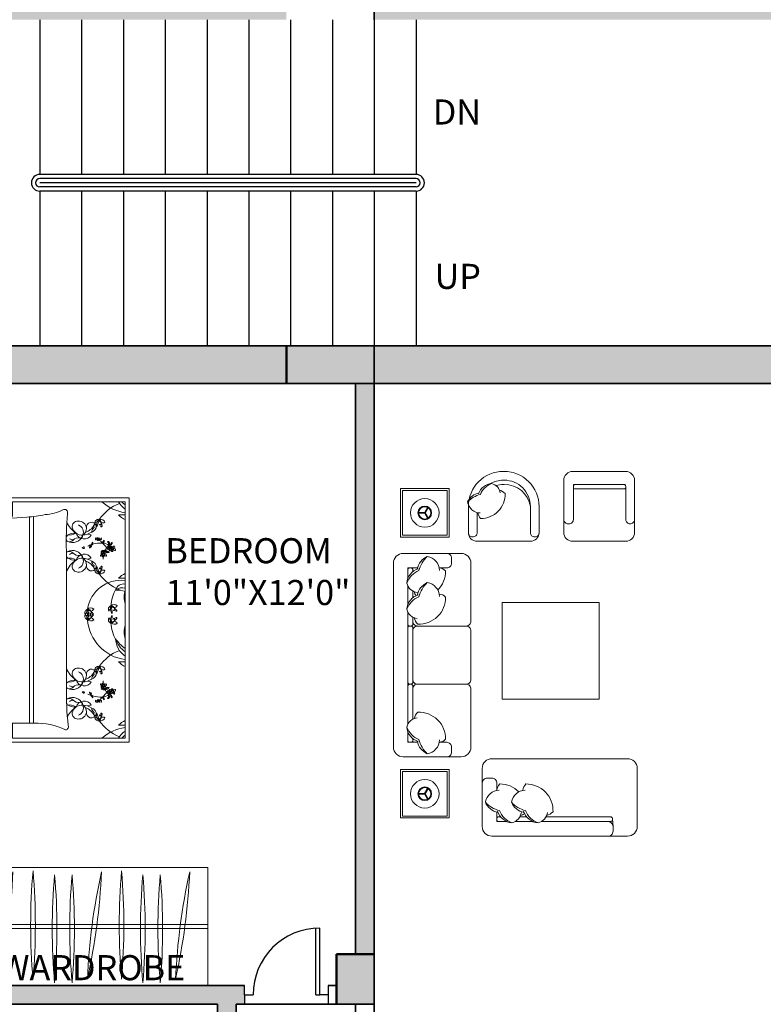
# Model space of a CAD drawing. Units: inches. Extents: x -28 to 485, y -861 to 54.
# Tile 3 of 14: x 76 to 254, y -600 to -365. Entities that reach past the tile are written whole.
import ezdxf

# ---------------------------------------------------------------- set-up
doc = ezdxf.new("R2010")
doc.units = ezdxf.units.IN
doc.header["$MEASUREMENT"] = 0
for name, color, linetype, lineweight in [('A-ANNO-TEXT', 7, 'Continuous', 18), ('A-AREA-IDEN', 7, 'Continuous', 18), ('A-COLS', 7, 'Continuous', 50), ('A-COLS-PATT', 8, 'Continuous', 13), ('A-DOOR', 3, 'Continuous', 25), ('A-FLOR-CASE', 8, 'Continuous', 18), ('A-FLOR-STRS', 7, 'Continuous', 25), ('A-FURN', 8, 'Continuous', 13), ('A-WALL', 7, 'Continuous', 35), ('A-WALL-PATT', 34, 'Continuous', 13)]:
    doc.layers.add(name, color=color, linetype=linetype, lineweight=lineweight)
doc.styles.get("Standard").update_dxf_attribs({"font": 'arial.ttf'})

# ---------------------------------------------------------------- blocks, each defined once
blk = doc.blocks.new('DAY BED1')
at = {"color": 0}
blk.add_line((0.3, 0.25), (0.225, 0.255), dxfattribs=at)
blk.add_lwpolyline([(-0.3, 0, -0.414214), (-0.4, 0.1), (-0.4, 0.1, 0.317837), (-0.4, 0.1, -0.414214), (-0.4, 0.1), (-0.4, 0.1, 1.186185), (-0.4, 0.1, -0.414214), (-0.4, 0.1), (-0.4, 1.5, -0.414214), (-0.3, 1.6), (0.3, 1.6, -0.414214), (0.4, 1.5), (0.4, 0.1, -0.414214), (0.3, 0)], format="xyb", close=True, dxfattribs=at)
for points in [[(-0.073, 1.45), (-0.15, 1.45, -0.414214), (-0.2, 1.5), (-0.2, 1.55, -0.414214), (-0.15, 1.6)], [(-0.076, 1.425, -0.356772), (0.05, 1.568, -0.249542), (0.154, 1.438, 9.61688)], [(0.05, 1.568, -0.14773), (0.136, 1.422, -0.213343), (0.262, 1.293, -0.178662)], [(-0.073, 1.45, 0.165541), (-0.139, 1.419, 0.200231), (-0.058, 1.221, 0.121523)], [(0.143, 1.442, -0.306663), (0.262, 1.293, -0.30633), (0.154, 1.196, 0.872847)], [(0.25, 1.345), (0.25, 1.45), (0.152, 1.45, -0.414214)], [(0.2, 1.412), (0.2, 1.43, -0.414214), (0.22, 1.45), (0.23, 1.45, -0.414214), (0.25, 1.43)], [(0.25, 1.43), (0.25, 1.345, -0.414214)], [(-0.076, 1.156, -0.356772), (0.05, 1.299, -0.249542), (0.154, 1.169, 9.61688)], [(0.05, 1.299, -0.14773), (0.136, 1.153, -0.213343), (0.262, 1.024, -0.178662)], [(0.25, 1.262), (0.25, 1.075, -0.414214)], [(-0.073, 1.181, 0.165541), (-0.139, 1.15, 0.425989), (0.148, 0.869, 0.121523), (0.187, 0.936, -7.115464)], [(0.143, 1.173, -0.306663), (0.262, 1.024, -0.30633), (0.154, 0.926, 0.872847)], [(0.168, 1.163, 0.071865), (0.187, 1.205, -7.115464)], [(0.2, 1.142), (0.2, 1.211, -0.414214)], [(0.25, 0.992), (0.25, 0.275, -0.414214), (0.23, 0.255), (0.22, 0.255, -0.414214), (0.2, 0.275), (0.2, 0.942, -0.414214)], [(0.25, 0.377), (0.25, 0.3, 0.414214), (0.3, 0.25), (0.35, 0.25, 0.414214), (0.4, 0.3)]]:
    blk.add_lwpolyline(points, format="xyb", dxfattribs=at)
for points in [[(0.25, 1.075), (0.25, 1.262)], [(0.25, 0.377), (0.25, 0.992)]]:
    blk.add_lwpolyline(points, dxfattribs=at)
blk = doc.blocks.new('BED-DOUBLE-WITH-NIGHTSTANDS')
for p, q in [((0, 0), (0, 80.08)), ((6.67, 66.84), (6.67, 77.31)), ((11.91, 72.08), (1.44, 72.08)), ((39.26, 64.51), (39.26, 68.96)), ((39.26, 68.96), (68.11, 68.96)), ((68.11, 68.96), (68.11, 10.57)), ((40.19, 68.03), (40.19, 64.5)), ((67.18, 68.03), (40.19, 68.03)), ((67.18, 11.5), (67.18, 68.03)), ((1.03, 64.07), (1.03, 16.02)), ((12.66, 16.02), (12.66, 64.07)), ((15.98, 63.85), (16.38, 35.34)), ((16.8, 63.82), (17.22, 34.74)), ((19.33, 63.78), (19.45, 33.37)), ((20.15, 63.78), (20.27, 33.06)), ((44.25, 64.43), (44.25, 15.09)), ((45.25, 64.51), (45.25, 15.09)), ((59.06, 60.14), (58.15, 60.31)), ((53.12, 56.3), (53.12, 23.78)), ((59.06, 54.54), (58.15, 54.36)), ((12.66, 38.02), (18.76, 33.63)), ((15.04, 27.14), (12.66, 35.87)), ((18.76, 33.63), (23.47, 31.84)), ((23.47, 31.84), (25.57, 31.52)), ((25.57, 31.52), (24.92, 28.93)), ((24.92, 28.93), (23.95, 26.82)), ((17.14, 21.3), (15.04, 27.14)), ((23.95, 26.82), (23.47, 23.25)), ((59.06, 24.99), (58.15, 25.16)), ((19.41, 18.22), (17.14, 21.3)), ((23.47, 23.25), (23.14, 19.19)), ((23.14, 19.19), (23.47, 15.95)), ((59.06, 19.39), (58.15, 19.21)), ((22.82, 15.3), (19.41, 18.22)), ((0, 16.02), (21.98, 16.02)), ((23.47, 15.95), (22.82, 15.3)), ((39.26, 10.57), (39.26, 15.1)), ((40.19, 15.1), (40.19, 11.5)), ((6.67, 13.24), (6.67, 2.78)), ((68.11, 10.57), (39.26, 10.57)), ((40.19, 11.5), (67.18, 11.5)), ((11.91, 8.01), (1.44, 8.01))]:
    blk.add_line(p, q)
for points in [[(0, 64.07), (13.35, 64.07), (13.35, 80.08), (0, 80.08)], [(6.67, 72.08), (5.06, 71.14)], [(6.67, 72.08), (8.29, 71.14)], [(13.35, 16.02), (13.35, 0), (0, 0)], [(6.67, 8.01), (5.06, 8.94)], [(6.67, 8.01), (8.29, 8.94)]]:
    blk.add_lwpolyline(points)
for points in [[(43.62, 64.41, 0.056112), (48.03, 64.99, 0.095341), (52.27, 66.12)], [(2, 59.47, -0.074897), (7.23, 59.37, 0.472817)], [(7.52, 43.09, -0.14099), (2.18, 42.93, -0.235245)], [(7.52, 39.67, 0.14099), (2.18, 39.83, 0.235245)], [(2, 20.62, 0.074897), (7.23, 20.71, -0.472817)], [(30.15, 15.13, 0.001242), (45.35, 15.09, -0.127202), (52.92, 13.49)]]:
    blk.add_lwpolyline(points, format="xyb")
for centre, radius in [((6.67, 72.08), 3.74), ((6.67, 72.08), 1.87), ((64.11, 56.84), 0.204), ((61.96, 55.51), 0.204), ((61.96, 24.02), 0.204), ((64.11, 22.68), 0.204), ((6.67, 8.01), 3.74), ((6.67, 8.01), 1.87)]:
    blk.add_circle(centre, radius)
for centre, radius, start, end in [((52.68, 65.51), 0.73, 336.5219, 123.8264), ((69.62, 57.92), 10.46, 111.4092, 145.6135), ((68.59, 75.81), 10.46, 228.1144, 262.255), ((69.99, 70.57), 5.1, 209.8884, 236.5383), ((70.94, 72.4), 6.35, 223.5186, 233.6964), ((22.44, 207.63), 143.9, 266.1, 270.9282), ((27.68, 251.44), 187.71, 269.1145, 274.8735), ((131.01, 58.75), 77.93, 175.2402, 181.8035), ((60.79, 62.99), 0.867, 76.272, 177.0484), ((59.47, 64.76), 1.79, 284.7031, 328.6173), ((61.96, 62.49), 1.65, 125.7657, 194.5347), ((53.85, 65.41), 7.32, 332.8176, 347.4827), ((61.24, 62.69), 1.16, 20.9613, 102.2885), ((61.86, 63.85), 0.873, 181.7131, 301.5367), ((59, 62.09), 2.64, 2.0648, 41.1598), ((60.59, 63.07), 0.856, 316.2238, 62.3173), ((68.81, 67.71), 4.25, 221.0454, 247.4453), ((66.52, 79.36), 14.47, 266.3481, 272.5919), ((58.76, 65.61), 6.06, 203.6453, 236.3329), ((55.85, 62.08), 1.35, 88.9462, 185.5144), ((56.85, 62.5), 2.41, 193.079, 274.7067), ((56.04, 61.53), 1.91, 7.1143, 95.0551), ((55.32, 60.77), 1.86, 338.5779, 68.4181), ((55.62, 61.86), 2.33, 305.9599, 357.6409), ((56.48, 64.35), 3.78, 288.2955, 328.7386), ((59.12, 61.97), 1.2, 19.1312, 189.736), ((58.76, 62.26), 1.5, 285.6955, 4.031), ((60.76, 60.64), 1.6, 128.4175, 173.8338), ((60.43, 62.21), 0.737, 126.7319, 206.0245), ((61.09, 62.57), 0.0682, 20.2667, 316.2271), ((61.51, 62.18), 0.13, 168.5166, 2.0648), ((61.45, 62.19), 0.0631, 52.0591, 168.5166), ((-760.15, 15.33), 763.42, 2.85022, 3.31479), ((9.33, 49.26), 10.32, 78.2417, 114.8684), ((1.06, 56.61), 10.73, 348.9631, 14.8961), ((54, 59.28), 0.964, 127.675, 162.5814), ((54, 59.28), 0.964, 196.6343, 225.5483), ((53.71, 63.39), 3.32, 259.249, 301.1782), ((54.57, 60.82), 2.55, 240.8249, 340.7178), ((53.81, 59.69), 1.2, 246.1646, 318.4347), ((55.15, 57.49), 3.09, 85.2696, 124.215), ((55.03, 61.2), 2.3, 240.0851, 262.564), ((55.94, 57.8), 1.64, 74.8529, 138.4347), ((57.33, 61.13), 1.99, 196.8663, 330.0915), ((56.5, 59.87), 0.497, 254.8529, 12.6959), ((55.15, 57.49), 3.09, 53.6555, 57.2989), ((56.78, 64.39), 4.3, 273.4924, 303.7117), ((60.19, 59.12), 0.158, 125.0752, 284.7644), ((60.43, 59.18), 0.34, 127.3642, 168.4363), ((60.17, 59.45), 0.49, 277.4968, 341.2737), ((60.56, 59.22), 0.195, 88.1325, 178.8919), ((60.95, 59.02), 0.422, 136.3462, 189.6513), ((60.71, 58.98), 0.176, 189.6513, 312.3208), ((60.75, 59.46), 0.204, 183.2768, 356.7232), ((61.39, 59.1), 0.668, 164.2829, 186.9148), ((60.6, 59.09), 0.334, 312.3208, 40.2111), ((61.31, 59.47), 0.474, 201.6382, 274.947), ((60.68, 58.82), 0.619, 42.3896, 66.5724), ((66.93, 63.72), 7.6, 217.9541, 226.8459), ((61.13, 59.18), 0.337, 10.9597, 52.2379), ((61.33, 59.15), 0.156, 274.947, 37.5263), ((57.16, 57.12), 0.251, 169.5864, 349.5616), ((57.25, 57.11), 0.154, 349.5616, 167.2949), ((61.28, 51.56), 6.63, 110.1059, 116.9968), ((59.06, 57.02), 0.42, 129.5056, 182.6421), ((57.85, 58), 1.27, 308.4388, 328.836), ((57.63, 59.02), 2.26, 296.5064, 305.3102), ((57.61, 57.86), 1.29, 336.3901, 344.4871), ((59.01, 57.53), 0.163, 83.9457, 185.6216), ((58.36, 57.69), 0.671, 328.836, 0.8141), ((58.71, 57.49), 0.384, 306.5232, 32.4668), ((59.16, 57.79), 0.163, 112.5583, 214.2343), ((59.06, 58.08), 0.384, 265.7131, 351.6568), ((58.72, 58.29), 0.671, 297.3659, 329.344), ((58.21, 58.87), 1.29, 313.6929, 321.7899), ((59.64, 57.99), 0.42, 115.5379, 168.6744), ((58.21, 58.6), 1.27, 329.344, 349.7412), ((61.28, 51.56), 6.63, 86.1723, 106.4158), ((57.2, 58.31), 2.26, 352.8698, 1.6736), ((61.66, 57.07), 0.93, 253.6301, 325.4631), ((61.86, 58.27), 0.163, 112.5583, 214.2343), ((61.75, 58.56), 0.384, 265.7131, 351.6568), ((61.42, 58.77), 0.671, 297.3659, 329.344), ((61.45, 54.86), 3.33, 60.7959, 85.244), ((54.37, 50.07), 10.94, 37.8256, 47.7588), ((60.91, 59.35), 1.29, 313.6929, 321.7899), ((61.87, 56.57), 0.565, 273.8774, 357.1501), ((62.33, 58.47), 0.42, 115.5379, 168.6744), ((60.9, 59.07), 1.27, 329.344, 349.7412), ((62.09, 56.97), 0.547, 262.0748, 308.2393), ((59.89, 58.78), 2.26, 352.8698, 1.6736), ((62.87, 56.86), 0.547, 215.1128, 261.2773), ((63.31, 56.83), 0.93, 197.889, 269.722), ((65.87, 54.52), 3.99, 130.182, 149.456), ((63.07, 58.33), 0.228, 33.0979, 123.1364), ((58.05, 55.12), 5.96, 31.1156, 34.8118), ((62.74, 57.94), 0.617, 2.3172, 70.5201), ((63.67, 56.79), 0.658, 139.3812, 199.9959), ((62.44, 57.27), 0.93, 310.9365, 22.7695), ((62.87, 57.22), 0.675, 285.6484, 332.2957), ((63.25, 57.78), 0.178, 135.7354, 318.1297), ((62.95, 58.07), 0.236, 315.7354, 31.1156), ((62.75, 57.57), 0.547, 319.3812, 5.5456), ((63.38, 57.79), 0.178, 68.2452, 250.6395), ((62.97, 58), 0.531, 352.6008, 57.1845), ((64.87, 54.44), 3.55, 111.7087, 116.2181), ((61.45, 54.86), 3.33, 47.5083, 55.9967), ((63.48, 58.12), 0.531, 252.8042, 349.6943), ((62.97, 57.17), 0.565, 331.1838, 51.6792), ((63.55, 56.5), 0.158, 125.0752, 284.7644), ((63.53, 58.17), 0.236, 248.2452, 323.6254), ((63.8, 56.56), 0.34, 93.635, 168.4363), ((63.33, 58.31), 0.617, 291.7087, 3.0299), ((63.75, 57.1), 0.2, 138.2946, 276.2474), ((63.53, 56.83), 0.49, 277.4968, 341.2737), ((63.83, 57.07), 0.278, 358.5719, 143.8954), ((58.93, 61.56), 5.96, 323.6254, 327.3216), ((63.92, 56.61), 0.195, 88.1325, 178.8919), ((63.99, 57.29), 0.281, 208.8493, 269.9355), ((63.75, 57.22), 0.321, 274.2123, 318.1587), ((64.31, 56.4), 0.422, 136.3462, 189.6513), ((63.81, 58.16), 0.228, 325.6077, 55.6462), ((64.75, 56.48), 0.668, 164.2829, 186.9148), ((64.73, 56.9), 0.643, 121.9501, 165.2442), ((63.96, 56.47), 0.334, 312.3208, 40.2111), ((64.67, 56.85), 0.474, 201.6382, 274.947), ((64.28, 57.14), 0.135, 262.868, 7.094), ((64.04, 56.2), 0.619, 42.3896, 66.5724), ((64.27, 57.26), 0.403, 278.5614, 22.5914), ((64.49, 56.56), 0.337, 10.9597, 118.7804), ((64.49, 57.27), 0.202, 44.3732, 121.9501), ((64.7, 56.53), 0.156, 274.947, 37.5263), ((1.85, 51.98), 10.19, 333.8761, 16.1746), ((54, 55.39), 0.964, 134.4517, 156.7144), ((54, 55.39), 0.964, 203.2856, 232.325), ((53.71, 51.28), 3.32, 58.8218, 100.2867), ((54.57, 53.85), 2.55, 19.2822, 119.1751), ((53.81, 54.99), 1.2, 41.5653, 113.8354), ((55.15, 57.18), 3.09, 235.785, 274.7304), ((55.03, 53.47), 2.3, 97.436, 119.9149), ((56.85, 52.18), 2.41, 85.2933, 166.921), ((55.94, 56.87), 1.64, 221.5653, 285.1471), ((57.33, 53.55), 1.99, 29.9085, 163.1337), ((55.32, 53.9), 1.86, 291.5819, 21.4221), ((56.5, 54.81), 0.497, 347.3041, 105.1471), ((55.15, 57.18), 3.09, 302.7011, 306.3445), ((55.62, 52.81), 2.33, 2.3591, 54.0401), ((56.78, 50.29), 4.3, 56.2883, 86.5076), ((61.4, 55.17), 0.158, 125.0752, 284.7644), ((61.65, 55.23), 0.34, 93.635, 168.4363), ((61.92, 55.78), 0.658, 82.0748, 142.6895), ((61.85, 56.68), 0.675, 228.342, 274.9894), ((61.6, 55.76), 0.2, 138.2946, 276.2474), ((61.38, 55.5), 0.49, 277.4968, 341.2737), ((61.68, 55.73), 0.278, 358.5719, 143.8954), ((61.77, 55.27), 0.195, 88.1325, 178.8919), ((61.84, 55.95), 0.281, 208.8493, 269.9355), ((61.6, 55.89), 0.321, 274.2123, 318.1587), ((62.16, 55.06), 0.422, 136.3462, 189.6513), ((61.92, 55.02), 0.176, 189.6513, 312.3208), ((65.87, 54.52), 3.99, 175.2415, 182.8929), ((62.6, 55.14), 0.668, 164.2829, 186.9148), ((62.58, 55.56), 0.643, 121.9501, 165.2442), ((61.81, 55.14), 0.334, 312.3208, 40.2111), ((62.52, 55.52), 0.474, 201.6382, 274.947), ((62.13, 55.81), 0.135, 262.868, 7.094), ((61.89, 54.87), 0.619, 42.3896, 66.5724), ((62.12, 55.92), 0.403, 278.5614, 22.5914), ((62.34, 55.23), 0.337, 10.9597, 118.7804), ((65.87, 54.52), 3.99, 156.1523, 156.9499), ((62.34, 55.94), 0.202, 44.3732, 121.9501), ((62.97, 56.41), 0.565, 181.4625, 249.4747), ((62.55, 55.2), 0.156, 274.947, 37.5263), ((63.02, 56.51), 0.675, 248.3627, 295.0101), ((62.69, 55.67), 0.658, 20.6625, 81.2773), ((64.07, 56.36), 0.176, 189.6513, 312.3208), ((16.01, 49.96), 14.08, 166.3427, 191.1841), ((58.76, 49.06), 6.06, 123.6671, 158.5059), ((55.85, 52.59), 1.35, 174.4856, 271.0538), ((56.04, 53.15), 1.91, 264.9449, 352.8857), ((56.48, 50.32), 3.78, 31.2614, 71.7045), ((59.12, 52.71), 1.2, 170.264, 340.8688), ((60.76, 54.03), 1.6, 186.1662, 231.5825), ((58.76, 52.42), 1.5, 355.969, 74.3045), ((60.43, 52.46), 0.737, 153.9755, 233.2681), ((61.96, 52.19), 1.65, 165.4653, 234.2343), ((53.85, 49.26), 7.32, 12.5173, 27.1824), ((59, 52.59), 2.64, 318.8402, 357.9352), ((60.59, 51.6), 0.856, 297.6827, 43.7762), ((61.13, 52.12), 0.113, 43.7762, 339.7183), ((61.51, 52.5), 0.13, 357.9352, 191.4834), ((61.45, 52.48), 0.0631, 191.4834, 307.9409), ((60.79, 51.69), 0.867, 182.9516, 283.728), ((59.47, 49.92), 1.79, 31.3827, 75.2969), ((61.86, 50.82), 0.873, 58.4633, 178.2869), ((61.24, 51.98), 1.16, 257.7115, 339.0387), ((69.62, 56.75), 10.46, 214.3865, 248.5908), ((68.81, 46.96), 4.25, 112.5547, 138.9546), ((66.52, 35.31), 14.47, 87.4081, 93.6519), ((66.17, 41.19), 8.09, 82.8636, 171.8197), ((74.19, 42.33), 10.46, 152.5854, 175.5377), ((66.74, 46.53), 1.88, 76.3898, 169.0739), ((66.48, 45.12), 2.37, 72.8609, 131.9049), ((5.99, 44.03), 3.96, 153.3437, 196.1026), ((7.37, 44.56), 4.25, 335.0183, 18.5407), ((65.43, 42.24), 4.68, 68.117, 96.6195), ((72.68, 45.26), 5.75, 162.9798, 196.4569), ((10.2, 52.53), 9.81, 254.1707, 275.9871), ((58.94, 41.49), 1.16, 50.8855, 132.2127), ((64.01, 42.31), 0.867, 106.1963, 206.9726), ((61.98, 43.19), 1.79, 314.6273, 358.5415), ((65.27, 42.46), 1.65, 155.6899, 224.4589), ((64.54, 42.29), 1.16, 50.8855, 132.2127), ((64.51, 43.6), 0.873, 211.6373, 331.4609), ((63.8, 42.29), 0.856, 346.148, 92.2415), ((62.91, 40.64), 2.64, 31.989, 71.0841), ((56.78, 40.96), 7.32, 2.7418, 17.407), ((75.64, 42.98), 8.5, 174.3643, 175.6213), ((81.47, 38.5), 15.2, 160.0972, 160.2783), ((10.2, 30.23), 9.81, 84.0129, 105.8293), ((58.4, 41.51), 0.867, 106.1963, 206.9726), ((58.4, 40.68), 0.867, 153.0274, 253.8037), ((56.38, 42.39), 1.79, 314.6273, 358.5415), ((56.38, 39.81), 1.79, 1.4585, 45.3727), ((59.67, 41.66), 1.65, 155.6899, 224.4589), ((59.67, 40.53), 1.65, 135.5411, 204.3101), ((58.91, 42.8), 0.873, 211.6373, 331.4609), ((58.2, 41.49), 0.856, 346.148, 92.2415), ((57.3, 39.84), 2.64, 31.989, 71.0841), ((51.18, 40.16), 7.32, 2.7418, 17.407), ((51.18, 42.04), 7.32, 342.593, 357.2582), ((57.3, 42.35), 2.64, 288.9159, 328.011), ((58.2, 40.71), 0.856, 267.7585, 13.852), ((58.91, 39.39), 0.873, 28.5391, 148.3627), ((58.87, 41.3), 0.0682, 50.1909, 346.0209), ((58.92, 40.88), 0.113, 13.852, 309.9245), ((59.44, 41.17), 0.13, 198.4408, 31.989), ((59.37, 41.15), 0.0631, 81.9833, 198.4408), ((59.44, 41.02), 0.13, 328.011, 161.5592), ((59.37, 41.04), 0.0631, 161.5592, 278.0167), ((64.01, 39.88), 0.867, 153.0274, 253.8037), ((61.98, 39.01), 1.79, 1.4585, 45.3727), ((65.27, 39.73), 1.65, 135.5411, 204.3101), ((56.78, 41.24), 7.32, 342.593, 357.2582), ((62.91, 41.55), 2.64, 288.9159, 328.011), ((63.8, 39.91), 0.856, 267.7585, 13.852), ((64.52, 40.08), 0.113, 13.852, 309.9245), ((64.47, 42.1), 0.0682, 50.1909, 346.0209), ((64.98, 41.95), 0.0631, 81.9833, 198.4408), ((64.98, 40.24), 0.0631, 161.5592, 278.0167), ((65.04, 41.98), 0.13, 198.4408, 31.989), ((65.04, 40.22), 0.13, 328.011, 161.5592), ((16.3, 37.72), 14.27, 171.5249, 193.96), ((-2.51, 36.66), 14.12, 349.8617, 13.6238), ((58.94, 40.71), 1.16, 227.7873, 309.1145), ((68.59, 40.66), 10.46, 184.4623, 262.255), ((64.51, 38.59), 0.873, 28.5391, 148.3627), ((64.54, 39.91), 1.16, 227.7873, 309.1145), ((74.19, 39.86), 10.46, 184.4623, 207.4146), ((72.68, 36.94), 5.75, 163.5431, 197.0202), ((75.64, 39.22), 8.5, 184.3787, 185.6357), ((81.47, 43.7), 15.2, 199.7217, 199.9028), ((30.98, 31.59), 29.04, 172.2196, 189.497), ((-6.57, 29.12), 18.61, 348.0397, 19.2615), ((69.99, 35.42), 5.1, 181.272, 236.5383), ((72.72, 40.59), 9.45, 214.0123, 234.053), ((70.94, 37.25), 6.35, 197.8504, 233.6964), ((-4.69, 37.08), 31.06, 340.1194, 349.3383), ((25.64, 31.34), 0.193, 358.8623, 109.7536), ((69.62, 22.77), 10.46, 111.4092, 145.6135), ((55.85, 26.93), 1.35, 88.9462, 185.5144), ((56.04, 26.38), 1.91, 7.1143, 95.0551), ((60.79, 27.84), 0.867, 76.272, 177.0484), ((59.47, 29.61), 1.79, 284.7031, 328.6173), ((61.96, 27.34), 1.65, 125.7657, 194.5347), ((53.85, 30.27), 7.32, 332.8176, 347.4827), ((61.24, 27.55), 1.16, 20.9613, 102.2885), ((60.59, 27.92), 0.856, 316.2238, 62.3173), ((59, 26.94), 2.64, 2.0648, 41.1598), ((61.86, 28.71), 0.873, 181.7131, 301.5367), ((66.52, 44.21), 14.47, 266.3481, 272.5919), ((68.81, 32.56), 4.25, 221.0454, 247.4453), ((-760.15, 64.76), 763.42, 356.68521, 357.14978), ((30.48, 23.89), 6.52, 156.2616, 191.3392), ((58.76, 30.46), 6.06, 201.4941, 236.3329), ((56.85, 27.35), 2.41, 193.079, 274.7067), ((55.32, 25.63), 1.86, 338.5779, 68.4181), ((55.62, 26.71), 2.33, 305.9599, 357.6409), ((56.48, 29.2), 3.78, 288.2955, 328.7386), ((59.12, 26.82), 1.2, 19.1312, 189.736), ((58.76, 27.11), 1.5, 285.6955, 4.031), ((60.76, 25.49), 1.6, 128.4175, 173.8338), ((60.43, 27.07), 0.737, 126.7319, 206.0245), ((61.09, 27.42), 0.0682, 20.2667, 316.2271), ((61.51, 27.03), 0.13, 168.5166, 2.0648), ((61.45, 27.04), 0.0631, 52.0591, 168.5166), ((1.06, 23.47), 10.73, 345.1039, 11.0369), ((136.48, 22.83), 83.37, 179.3433, 185.6887), ((53.71, 28.24), 3.32, 259.7133, 301.1782), ((54, 24.13), 0.964, 127.675, 156.7144), ((54, 24.13), 0.964, 203.229, 225.5483), ((54.57, 25.67), 2.55, 240.8249, 340.7178), ((53.81, 24.54), 1.2, 246.1646, 318.4347), ((55.15, 22.34), 3.09, 85.2696, 124.215), ((55.03, 26.06), 2.3, 240.0851, 262.564), ((55.94, 22.65), 1.64, 74.8529, 138.4347), ((57.33, 25.98), 1.99, 196.8663, 330.0915), ((56.5, 24.72), 0.497, 254.8529, 12.6959), ((55.15, 22.34), 3.09, 53.6555, 57.2989), ((56.78, 29.24), 4.3, 273.4924, 303.7117), ((61.4, 24.36), 0.158, 75.2356, 234.9248), ((61.65, 24.3), 0.34, 191.5637, 266.365), ((61.6, 23.76), 0.2, 83.7526, 221.7054), ((61.38, 24.03), 0.49, 18.7263, 82.5032), ((61.68, 23.79), 0.278, 216.1046, 1.4281), ((61.77, 24.25), 0.195, 181.1081, 271.8675), ((61.84, 23.57), 0.281, 90.0645, 151.1507), ((61.6, 23.64), 0.321, 41.8413, 85.7877), ((61.92, 24.5), 0.176, 47.6792, 170.3487), ((62.16, 24.46), 0.422, 170.3487, 223.6538), ((65.87, 25.01), 3.99, 177.1071, 184.7585), ((62.6, 24.38), 0.668, 173.0852, 195.7171), ((62.58, 23.96), 0.643, 194.7558, 238.0499), ((61.81, 24.39), 0.334, 319.7889, 47.6792), ((62.52, 24.01), 0.474, 85.053, 158.3618), ((62.13, 23.71), 0.135, 352.906, 97.132), ((61.89, 24.66), 0.619, 293.4276, 317.6104), ((62.34, 24.29), 0.337, 241.2196, 349.0403), ((62.12, 23.6), 0.403, 337.4086, 81.4386), ((62.97, 23.11), 0.565, 110.5253, 178.5375), ((63.31, 22.7), 0.93, 90.278, 162.111), ((62.55, 24.33), 0.156, 322.4737, 85.053), ((63.02, 23.01), 0.675, 64.9899, 111.6373), ((62.69, 23.86), 0.658, 278.7227, 339.3375), ((9.33, 30.82), 10.32, 245.1316, 281.7583), ((-5.54, 16.67), 30.23, 357.4519, 11.3392), ((54.57, 18.71), 2.55, 19.2822, 119.1751), ((57.16, 22.4), 0.251, 10.4384, 190.4136), ((57.25, 22.42), 0.154, 192.7051, 10.4384), ((61.28, 27.97), 6.63, 243.0032, 249.8941), ((57.85, 21.53), 1.27, 31.164, 51.5612), ((59.06, 22.5), 0.42, 177.3579, 230.4944), ((57.63, 20.5), 2.26, 54.6898, 63.4936), ((57.61, 21.66), 1.29, 15.5129, 23.6099), ((59.01, 21.99), 0.163, 174.3784, 276.0543), ((58.71, 22.03), 0.384, 327.5332, 53.4768), ((58.36, 21.84), 0.671, 359.1859, 31.164), ((59.16, 21.74), 0.163, 145.7657, 247.4417), ((59.06, 21.45), 0.384, 8.3432, 94.2869), ((58.72, 21.23), 0.671, 30.656, 62.6341), ((58.21, 20.66), 1.29, 38.2101, 46.3071), ((59.64, 21.53), 0.42, 191.3256, 244.4621), ((58.21, 20.93), 1.27, 10.2588, 30.656), ((61.28, 27.97), 6.63, 253.5842, 273.8277), ((57.2, 21.22), 2.26, 358.3264, 7.1302), ((66.93, 15.8), 7.6, 133.1541, 142.0459), ((61.85, 22.84), 0.675, 85.0106, 131.658), ((61.66, 22.46), 0.93, 34.5369, 106.3699), ((61.92, 23.75), 0.658, 217.3105, 277.9252), ((61.86, 21.26), 0.163, 145.7657, 247.4417), ((54.37, 29.45), 10.94, 312.2412, 322.1744), ((61.45, 24.67), 3.33, 274.756, 299.2041), ((61.75, 20.97), 0.384, 8.3432, 94.2869), ((61.42, 20.76), 0.671, 30.656, 62.6341), ((61.87, 22.95), 0.565, 2.8499, 86.1226), ((62.09, 22.55), 0.547, 51.7607, 97.9252), ((65.87, 25.01), 3.99, 203.0501, 203.8477), ((62.34, 23.59), 0.202, 238.0499, 315.6268), ((62.87, 22.67), 0.547, 98.7227, 144.8872), ((65.87, 25.01), 3.99, 210.544, 229.818), ((62.74, 21.59), 0.617, 289.4799, 357.6828), ((58.05, 24.41), 5.96, 325.1882, 328.8844), ((63.67, 22.74), 0.658, 160.0041, 220.6188), ((62.44, 22.26), 0.93, 337.2305, 49.0635), ((62.87, 22.31), 0.675, 27.7043, 74.3516), ((63.25, 21.74), 0.178, 41.8703, 224.2646), ((62.95, 21.45), 0.236, 328.8844, 44.2646), ((62.75, 21.95), 0.547, 354.4544, 40.6188), ((63.38, 21.74), 0.178, 109.3605, 291.7548), ((62.97, 21.52), 0.531, 302.8155, 7.3992), ((64.87, 25.09), 3.55, 243.7819, 248.2913), ((61.45, 24.67), 3.33, 304.0033, 312.4917), ((62.97, 22.35), 0.565, 308.3208, 28.8162), ((63.48, 21.4), 0.531, 10.3057, 107.1958), ((63.55, 23.03), 0.158, 75.2356, 234.9248), ((63.53, 21.36), 0.236, 36.3746, 111.7548), ((63.8, 22.96), 0.34, 191.5637, 266.365), ((63.75, 22.43), 0.2, 83.7526, 221.7054), ((63.33, 21.21), 0.617, 356.9701, 68.2913), ((63.53, 22.69), 0.49, 18.7263, 82.5032), ((63.83, 22.46), 0.278, 216.1046, 1.4281), ((63.92, 22.92), 0.195, 181.1081, 271.8675), ((58.93, 17.96), 5.96, 32.6784, 36.3746), ((63.99, 22.24), 0.281, 90.0645, 151.1507), ((63.75, 22.31), 0.321, 41.8413, 85.7877), ((64.07, 23.17), 0.176, 47.6792, 170.3487), ((64.31, 23.13), 0.422, 170.3487, 223.6538), ((63.81, 21.37), 0.228, 304.3538, 34.3923), ((64.75, 23.05), 0.668, 173.0852, 195.7171), ((64.73, 22.63), 0.643, 194.7558, 238.0499), ((63.96, 23.05), 0.334, 319.7889, 47.6792), ((64.67, 22.68), 0.474, 85.053, 158.3618), ((64.28, 22.38), 0.135, 352.906, 97.132), ((64.04, 23.32), 0.619, 293.4276, 317.6104), ((64.49, 22.96), 0.337, 241.2196, 349.0403), ((64.27, 22.27), 0.403, 337.4086, 81.4386), ((64.49, 22.25), 0.202, 238.0499, 315.6268), ((64.7, 22.99), 0.156, 322.4737, 85.053), ((54, 20.25), 0.964, 134.4517, 153.558), ((54, 20.25), 0.964, 210.0293, 232.325), ((53.71, 16.14), 3.32, 58.8218, 99.1554), ((53.81, 19.84), 1.2, 41.5653, 113.8354), ((58.76, 13.91), 6.06, 123.6671, 153.2997), ((55.15, 22.04), 3.09, 235.785, 274.7304), ((55.03, 18.32), 2.3, 97.436, 119.9149), ((56.85, 17.03), 2.41, 85.2933, 166.921), ((55.94, 21.72), 1.64, 221.5653, 285.1471), ((57.33, 18.4), 1.99, 29.9085, 163.1337), ((55.32, 18.75), 1.86, 291.5819, 21.4221), ((56.5, 19.66), 0.497, 347.3041, 105.1471), ((55.15, 22.04), 3.09, 302.7011, 306.3445), ((55.62, 17.67), 2.33, 2.3591, 54.0401), ((56.78, 15.14), 4.3, 56.2883, 86.5076), ((60.19, 20.41), 0.158, 75.2356, 234.9248), ((60.43, 20.35), 0.34, 191.5637, 232.6358), ((60.17, 20.07), 0.49, 18.7263, 82.5032), ((60.56, 20.3), 0.195, 181.1081, 271.8675), ((60.71, 20.55), 0.176, 47.6792, 170.3487), ((60.95, 20.51), 0.422, 170.3487, 223.6538), ((60.75, 20.06), 0.204, 3.2768, 176.7232), ((61.39, 20.43), 0.668, 173.0852, 195.7171), ((60.6, 20.43), 0.334, 319.7889, 47.6792), ((61.31, 20.06), 0.474, 85.053, 158.3618), ((60.68, 20.7), 0.619, 293.4276, 317.6104), ((61.13, 20.34), 0.337, 307.7621, 349.0403), ((61.33, 20.37), 0.156, 322.4737, 85.053), ((60.91, 20.18), 1.29, 38.2101, 46.3071), ((62.33, 21.06), 0.42, 191.3256, 244.4621), ((60.9, 20.45), 1.27, 10.2588, 30.656), ((59.89, 20.74), 2.26, 358.3264, 7.1302), ((63.07, 21.2), 0.228, 236.8636, 326.9021), ((55.85, 17.44), 1.35, 174.4856, 271.0538), ((56.04, 18), 1.91, 264.9449, 352.8857), ((56.48, 15.18), 3.78, 31.2614, 71.7045), ((59.12, 17.56), 1.2, 170.264, 340.8688), ((58.76, 17.27), 1.5, 355.969, 74.3045), ((60.76, 18.89), 1.6, 186.1662, 231.5825), ((60.43, 17.31), 0.737, 153.9755, 233.2681), ((59.47, 14.77), 1.79, 31.3827, 75.2969), ((60.79, 16.54), 0.867, 182.9516, 283.728), ((61.96, 17.04), 1.65, 165.4653, 234.2343), ((53.85, 14.11), 7.32, 12.5173, 27.1824), ((59, 17.44), 2.64, 318.8402, 357.9352), ((60.59, 16.46), 0.856, 297.6827, 43.7762), ((61.86, 15.67), 0.873, 58.4633, 178.2869), ((61.13, 16.97), 0.113, 43.7762, 339.7183), ((61.51, 17.35), 0.13, 357.9352, 191.4834), ((61.45, 17.33), 0.0631, 191.4834, 307.9409), ((24.81, -58.13), 73.46, 85.8294, 91.553), ((52.87, 14.23), 0.739, 273.98, 27.3412), ((61.24, 16.83), 1.16, 257.7115, 339.0387), ((69.62, 21.6), 10.46, 214.3865, 248.5908), ((68.81, 11.81), 4.25, 112.5547, 138.9546), ((66.52, 0.17), 14.47, 87.4081, 93.6519), ((68.59, 3.71), 10.46, 97.745, 131.8856), ((69.99, 8.96), 5.1, 123.4617, 150.1116), ((70.94, 7.13), 6.35, 126.3036, 136.4814)]:
    blk.add_arc(centre, radius, start, end)
blk = doc.blocks.new('WARDROBE-HANGING')
for p, q in [((84.7, 28.23), (0, 28.23)), ((0, 28.23), (0, 0)), ((84.7, 28.23), (84.7, 0)), ((84.7, 14.59), (0, 14.59)), ((84.7, 13.65), (0, 13.65)), ((84.7, 0), (0, 0))]:
    blk.add_line(p, q)
for centre, start, end in [((153.74, 13.55), 175.0028, 184.9972), ((-142.25, 13.55), 355.0028, 4.9972), ((157.93, 13.55), 175.0028, 184.9972), ((-138.07, 13.55), 355.0028, 4.9972), ((-131.46, 33.65), 347.508, 357.5023), ((162.01, -4.96), 167.508, 177.5023), ((169.76, 14.46), 175.0028, 184.9972), ((-126.23, 14.46), 355.0028, 4.9972), ((174.85, 13.55), 175.0028, 184.9972), ((-121.15, 13.55), 355.0028, 4.9972), ((179.03, 13.55), 175.0028, 184.9972), ((-116.97, 13.55), 355.0028, 4.9972), ((-110.36, 33.65), 347.508, 357.5023), ((183.11, -4.96), 167.508, 177.5023), ((190.86, 14.46), 175.0028, 184.9972), ((-105.13, 14.46), 355.0028, 4.9972), ((196.03, 13.55), 175.0028, 184.9972), ((-99.97, 13.55), 355.0028, 4.9972), ((200.21, 13.55), 175.0028, 184.9972), ((-95.78, 13.55), 355.0028, 4.9972), ((204.29, -4.96), 167.508, 177.5023), ((-89.17, 33.65), 347.508, 357.5023), ((212.05, 14.46), 175.0028, 184.9972), ((-83.95, 14.46), 355.0028, 4.9972), ((217.13, 13.55), 175.0028, 184.9972), ((-78.86, 13.55), 355.0028, 4.9972), ((221.31, 13.55), 175.0028, 184.9972), ((-74.68, 13.55), 355.0028, 4.9972), ((225.4, -4.96), 167.508, 177.5023), ((-68.07, 33.65), 347.508, 357.5023)]:
    blk.add_arc(centre, 148.56, start, end)
blk = doc.blocks.new('TABLE-END-WITH-LAMP')
for p, q in [((5.73, 5.83), (6.55, 7.24)), ((5.86, 5.76), (6.67, 7.17)), ((5.79, 5.87), (4.16, 5.87)), ((5.79, 5.72), (4.16, 5.72)), ((5.73, 5.76), (6.55, 4.34)), ((5.86, 5.83), (6.67, 4.41))]:
    blk.add_line(p, q)
at = {"ltscale": 0.03}
blk.add_lwpolyline([(11.59, 0), (11.59, 11.58), (0, 11.58), (0, 0)], close=True, dxfattribs=at)
blk.add_lwpolyline([(11.12, 11.12), (11.12, 0.46), (0.46, 0.46), (0.46, 11.12)], close=True)
for radius in [3.42, 1.64, 1.47]:
    blk.add_circle((5.79, 5.79), radius)
blk = doc.blocks.new('TABLE-COFFEE-SQUARE')
at = {"ltscale": 0.03}
blk.add_lwpolyline([(23.17, 23.17), (23.17, 0), (0, 0), (0, 23.17)], close=True, dxfattribs=at)
blk = doc.blocks.new('DOOR-SWING-NARROW')
for p, q in [((17, 2.25), (17, 18.25)), ((18, 2.25), (18, 18.25)), ((0, 2.25), (0, 4.5)), ((20, 4.5), (20, 0)), ((0, 2.25), (0, 0)), ((0, 2.25), (2, 2.25)), ((17, 2.25), (18, 2.25)), ((20, 2.25), (18, 2.25))]:
    blk.add_line(p, q)
blk.add_arc((18, 2.25), 16, 90, 180)

msp = doc.modelspace()

# ---------------------------------------------------------------- hatches: boundary and pattern name
at = {"layer": 'A-COLS-PATT'}
h = msp.add_hatch(color=256, dxfattribs=at)
h.dxf.hatch_style = 1
h.paths.add_polyline_path([(441.285, -591.367), (420.285, -591.367), (420.285, -595.867), (420.285, -600.367), (441.285, -600.367)])
h.paths.add_polyline_path([(304.691, -588.367), (295.785, -588.367), (295.785, -600.367), (304.691, -600.367)])
h.paths.add_polyline_path([(160.785, -588.367), (151.785, -588.367), (151.785, -600.367), (160.785, -600.367)])
h.paths.add_polyline_path([(36.285, -591.367), (24.285, -591.367), (15.285, -591.367), (15.285, -600.367), (36.285, -600.367)])
h.paths.add_polyline_path([(36.285, -808.867), (15.285, -808.867), (15.285, -817.867), (36.285, -817.867)])
h.paths.add_polyline_path([(160.785, -808.867), (139.785, -808.867), (139.785, -817.867), (160.785, -817.867)])
h.paths.add_polyline_path([(316.785, -808.867), (295.785, -808.867), (295.785, -817.867), (316.785, -817.867)])
h.paths.add_polyline_path([(441.285, -808.867), (420.285, -808.867), (420.285, -817.867), (441.285, -817.867)])
h.paths.add_polyline_path([(36.285, -442.867), (15.285, -442.867), (15.285, -451.867), (36.285, -451.867)])
h.paths.add_polyline_path([(160.785, -442.867), (139.785, -442.867), (139.785, -451.867), (160.785, -451.867)])
h.paths.add_polyline_path([(316.785, -442.867), (295.785, -442.867), (295.785, -451.867), (316.785, -451.867)])
h.paths.add_polyline_path([(441.285, -442.867), (420.285, -442.867), (420.285, -451.867), (441.285, -451.867)])
at = {"layer": 'A-WALL-PATT'}
h = msp.add_hatch(color=256, dxfattribs=at)
h.dxf.hatch_style = 1
h.paths.add_polyline_path([(160.785, -808.867), (160.785, -817.867), (295.785, -817.867), (295.785, -808.867)])
h.paths.add_polyline_path([(316.785, -817.867), (323.776, -817.867), (323.776, -808.867), (316.785, -808.867)])
h.paths.add_polyline_path([(420.285, -817.867), (420.285, -808.867), (383.776, -808.867), (383.776, -817.867)])
h.paths.add_polyline_path([(432.285, -808.867), (441.285, -808.867), (441.285, -702.966), (432.285, -702.966), (432.285, -708.367), (397.785, -708.367), (397.785, -710.617), (397.785, -712.867), (432.285, -712.867)])
h.paths.add_polyline_path([(300.285, -712.867), (329.285, -712.867), (329.285, -710.617), (329.285, -708.367), (295.785, -708.367), (295.785, -808.867), (300.285, -808.867)])
h.paths.add_polyline_path([(160.785, -698.867), (158.535, -698.867), (156.285, -698.867), (156.285, -808.867), (160.785, -808.867)])
h.paths.add_polyline_path([(36.285, -808.867), (36.285, -817.867), (79.721, -817.867), (79.721, -808.867)])
h.paths.add_polyline_path([(15.285, -808.867), (24.285, -808.867), (24.285, -739.09), (15.285, -739.09)])
h.paths.add_polyline_path([(24.285, -640.781), (15.285, -640.781), (15.285, -679.09), (24.285, -679.09), (24.285, -664.867), (89.285, -664.867), (89.285, -662.617), (89.285, -660.367), (24.285, -660.367)])
h.paths.add_polyline_path([(15.285, -616.781), (24.285, -616.781), (24.285, -600.367), (15.285, -600.367)])
h.paths.add_polyline_path([(36.285, -595.867), (36.285, -600.367), (123.285, -600.367), (123.285, -660.367), (117.285, -660.367), (117.285, -664.867), (156.285, -664.867), (156.285, -670.867), (160.785, -670.867), (160.785, -660.367), (127.785, -660.367), (127.785, -600.367), (129.785, -600.367), (129.785, -598.117), (129.785, -595.867)])
h.paths.add_polyline_path([(367.785, -664.867), (363.285, -664.867), (363.285, -708.367), (357.285, -708.367), (357.285, -712.867), (369.785, -712.867), (369.785, -708.367), (367.785, -708.367)])
h.paths.add_polyline_path([(432.285, -664.867), (432.285, -666.966), (441.285, -666.966), (441.285, -642.367), (432.285, -642.367), (432.285, -660.367), (328.785, -660.367), (328.785, -664.867), (363.285, -664.867)])
h.paths.add_polyline_path([(333.285, -600.367), (420.285, -600.367), (420.285, -595.867), (326.785, -595.867), (326.785, -600.367), (328.785, -600.367), (328.785, -630.367), (331.035, -630.367), (333.285, -630.367)])
h.paths.add_polyline_path([(441.285, -600.367), (432.285, -600.367), (432.285, -618.367), (441.285, -618.367)])
h.paths.add_polyline_path([(432.285, -591.367), (441.285, -591.367), (441.285, -547.793), (432.285, -547.793)])
h.paths.add_polyline_path([(295.785, -588.367), (300.238, -588.367), (300.285, -583.867), (300.285, -451.867), (295.785, -451.867)])
h.paths.add_polyline_path([(420.285, -451.867), (420.285, -442.867), (316.785, -442.867), (316.785, -451.867)])
h.paths.add_polyline_path([(432.285, -487.793), (441.285, -487.793), (441.285, -451.867), (432.285, -451.867)])
h.paths.add_polyline_path([(432.285, -442.867), (441.285, -442.867), (441.285, -364.867), (432.285, -364.867)])
h.paths.add_polyline_path([(261.785, -451.867), (261.785, -447.367), (261.785, -444.758), (261.785, -442.867), (160.785, -442.867), (160.785, -451.867)])
h.paths.add_polyline_path([(139.785, -451.867), (139.785, -442.867), (36.285, -442.867), (36.285, -451.867)])
h.paths.add_polyline_path([(15.285, -491.617), (24.285, -491.617), (24.285, -451.867), (15.285, -451.867)])
h.paths.add_polyline_path([(24.285, -551.617), (15.285, -551.617), (15.285, -591.367), (24.285, -591.367)])
h.paths.add_polyline_path([(160.785, -451.867), (156.285, -451.867), (156.285, -588.367), (160.785, -588.367)])
h.paths.add_polyline_path([(139.785, -364.867), (139.785, -355.867), (36.285, -355.867), (36.285, -364.867)])
h.paths.add_polyline_path([(24.285, -364.867), (15.285, -364.867), (15.285, -373.867), (24.285, -373.867)])
h.paths.add_polyline_path([(15.285, -433.867), (15.285, -442.867), (24.285, -442.867), (24.285, -433.867)])
h.paths.add_polyline_path([(261.785, -364.867), (261.785, -360.367), (261.785, -355.867), (160.785, -355.867), (160.785, -364.867)])
h.paths.add_polyline_path([(295.785, -355.867), (289.785, -355.867), (289.785, -364.867), (295.785, -364.867)])
h.paths.add_polyline_path([(295.785, -355.867), (300.285, -355.867), (300.285, -259.867), (333.285, -259.867), (333.285, -257.617), (333.285, -255.367), (300.285, -255.367), (300.285, -207.367), (295.785, -207.367)])
h.paths.add_polyline_path([(420.285, -364.867), (420.285, -355.867), (316.785, -355.867), (316.785, -364.867)])
h.paths.add_polyline_path([(24.285, -311.192), (15.285, -311.192), (15.285, -355.867), (24.285, -355.867)])
h.paths.add_polyline_path([(24.285, -211.867), (54.144, -211.867), (54.144, -207.367), (24.285, -207.367), (24.285, -187.772), (15.285, -187.772), (15.285, -251.192), (24.285, -251.192)])
h.paths.add_polyline_path([(82.144, -207.367), (82.144, -209.617), (82.144, -211.867), (127.785, -211.867), (127.785, -147.367), (129.785, -147.367), (129.785, -145.117), (129.785, -142.867), (36.285, -142.867), (36.285, -147.367), (123.285, -147.367), (123.285, -207.367)])
h.paths.add_polyline_path([(160.785, -207.367), (156.285, -207.367), (156.285, -355.867), (160.785, -355.867)])
h.paths.add_polyline_path([(24.285, 1.133), (15.285, 1.133), (15.285, -54.408), (24.285, -54.408)])
h.paths.add_polyline_path([(36.285, 10.133), (36.285, 1.133), (70.235, 1.133), (70.235, 10.133)])
h.paths.add_polyline_path([(15.285, -138.367), (24.285, -138.367), (24.285, -114.408), (15.285, -114.408)])
h.paths.add_polyline_path([(24.285, -147.367), (15.285, -147.367), (15.285, -163.772), (24.285, -163.772)])
h.paths.add_polyline_path([(156.285, -130.867), (160.785, -130.867), (160.785, 1.133), (156.285, 1.133)])
h.paths.add_polyline_path([(130.235, 1.133), (139.785, 1.133), (139.785, 10.133), (130.235, 10.133)])
h.paths.add_polyline_path([(316.785, 10.133), (316.785, 1.133), (328.097, 1.133), (328.097, 10.133)])
h.paths.add_polyline_path([(300.285, 1.133), (295.785, 1.133), (295.785, -130.867), (300.285, -130.867)])
h.paths.add_polyline_path([(420.285, -147.367), (420.285, -142.867), (326.785, -142.867), (326.785, -145.117), (326.785, -147.367), (328.785, -147.367), (328.785, -177.367), (331.035, -177.367), (333.285, -177.367), (333.285, -147.367)])
h.paths.add_polyline_path([(333.285, -207.367), (333.285, -205.367), (328.785, -205.367), (328.785, -211.867), (363.285, -211.867), (363.285, -255.367), (361.285, -255.367), (361.285, -259.867), (369.785, -259.867), (369.785, -255.367), (367.785, -255.367), (367.785, -211.867), (432.285, -211.867), (432.285, -214.893), (441.285, -214.893), (441.285, -188.008), (432.285, -188.008), (432.285, -207.367)])
h.paths.add_polyline_path([(441.285, -250.893), (432.285, -250.893), (432.285, -255.367), (397.785, -255.367), (397.785, -257.617), (397.785, -259.867), (432.285, -259.867), (432.285, -355.867), (441.285, -355.867)])
h.paths.add_polyline_path([(432.285, -138.367), (441.285, -138.367), (441.285, -115.099), (432.285, -115.099)])
h.paths.add_polyline_path([(441.285, -147.367), (432.285, -147.367), (432.285, -164.008), (441.285, -164.008)])
h.paths.add_polyline_path([(420.285, 1.133), (420.285, 10.133), (388.097, 10.133), (388.097, 1.133)])
h.paths.add_polyline_path([(432.285, -55.099), (441.285, -55.099), (441.285, 1.133), (432.285, 1.133)])

# ---------------------------------------------------------------- linework, layer by layer
at = {"layer": 'A-COLS'}
for p, q in [((139.785, -451.867), (139.785, -442.867)), ((151.785, -600.367), (151.785, -588.367)), ((151.785, -588.367), (160.785, -588.367))]:
    msp.add_line(p, q, dxfattribs=at)
at = {"layer": 'A-FLOR-STRS'}
for p, q in [((80.785, -364.867), (80.785, -401.867)), ((90.785, -364.867), (90.785, -401.867)), ((100.785, -364.867), (100.785, -401.867)), ((110.785, -364.867), (110.785, -401.867)), ((120.785, -364.867), (120.785, -401.867)), ((130.785, -364.867), (130.785, -401.867)), ((140.785, -364.867), (140.785, -401.867)), ((150.785, -364.867), (150.785, -401.867)), ((160.785, -364.867), (160.785, -401.867)), ((170.785, -364.867), (170.785, -401.867)), ((170.785, -401.867), (80.785, -401.867)), ((170.785, -402.867), (80.785, -402.867)), ((170.785, -403.867), (80.785, -403.867)), ((170.785, -404.867), (80.785, -404.867)), ((170.785, -405.867), (80.785, -405.867)), ((80.785, -405.867), (80.785, -442.867)), ((90.785, -405.867), (90.785, -442.867)), ((100.785, -405.867), (100.785, -442.867)), ((110.785, -405.867), (110.785, -442.867)), ((120.785, -405.867), (120.785, -442.867)), ((130.785, -405.867), (130.785, -442.867)), ((140.785, -405.867), (140.785, -442.867)), ((150.785, -405.867), (150.785, -442.867)), ((160.785, -405.867), (160.785, -442.867)), ((170.785, -405.867), (170.785, -442.867))]:
    msp.add_line(p, q, dxfattribs=at)
for centre, radius, start, end in [((80.785, -403.867), 2, 90, 270), ((170.785, -403.867), 2, 270, 90), ((80.785, -403.867), 1, 90, 270), ((170.785, -403.867), 1, 270, 90)]:
    msp.add_arc(centre, radius, start, end, dxfattribs=at)
at = {"layer": 'A-FURN', "ltscale": 0.03}
msp.add_lwpolyline([(191.773, -489.63), (198.145, -489.63, 0.4142136), (200.234, -487.541), (200.234, -481.274, 0.4142136), (191.878, -472.918), (191.773, -472.918), (191.669, -472.918, 0.4142136), (183.312, -481.274), (183.312, -487.541, 0.4142136), (185.402, -489.63), (191.773, -489.63)], format="xyb", dxfattribs=at)
for points in [[(220.973, -472.918), (220.973, -472.918, -0.4142136), (223.062, -475.007), (223.062, -487.541, -0.4142136), (220.973, -489.63), (220.973, -489.63), (208.229, -489.63, -0.4142136), (206.14, -487.541), (206.14, -475.007, -0.4142136), (208.229, -472.918)], [(181.61, -541.177, 0.4142136), (183.927, -538.86), (183.927, -524.958, 0.4142136), (182.769, -523.799, 0.4142136), (183.927, -522.641), (183.927, -511.056, 0.4142136), (182.769, -509.897, 0.4142136), (183.927, -508.739), (183.927, -494.837, 0.4142136), (181.61, -492.52), (167.708, -492.52, 0.4142136), (165.391, -494.837), (165.391, -538.86, 0.4142136), (167.708, -541.177)]]:
    msp.add_lwpolyline(points, format="xyb", close=True, dxfattribs=at)
at = {"layer": 'A-FURN'}
for points in [[(188.558, -475.833, -0.1305915), (191.669, -475.007), (191.773, -475.007)], [(198.145, -481.274, 0.4142136), (191.878, -475.007), (191.773, -475.007)], [(183.142, -480.22, -0.1477299), (186.195, -478.424, -0.2133428), (188.888, -475.792, -0.1786618)], [(186.135, -482.853, -0.3567724), (183.142, -480.22, -0.2495421), (185.854, -478.05, 9.6168803)], [(185.608, -482.789, 0.1655406), (186.254, -484.169, 0.4259892), (192.121, -478.185, 0.1215233), (190.728, -477.36, -7.1154643)], [(185.773, -478.281, -0.3066635), (188.888, -475.792, -0.30633), (190.924, -478.065, 0.8728472)], [(189.888, -476.276, -0.0723842), (191.669, -476.051), (191.773, -476.051)], [(198.145, -481.274, 0.3727189), (191.878, -476.051), (191.773, -476.051)], [(213.425, -477.096), (208.856, -477.096, -0.4142136), (208.438, -476.678), (208.438, -476.469, -0.4142136), (208.856, -476.051)], [(208.856, -476.051), (212.373, -476.051, -0.4142136)], [(212.373, -476.051), (220.555, -476.051, -0.4142136), (220.973, -476.469), (220.973, -476.678, -0.4142136), (220.555, -477.096), (213.425, -477.096, -0.4142136)], [(220.973, -476.678), (220.973, -484.408, 0.4142136), (222.017, -485.452), (222.017, -485.452, 0.4142136), (223.062, -484.408)], [(185.402, -482.739), (185.402, -487.541, -0.4142136), (184.357, -488.586), (184.357, -488.586, -0.4142136), (183.312, -487.541)], [(198.145, -481.274), (198.145, -487.541, 0.4142136), (199.19, -488.586), (199.19, -488.586, 0.4142136), (200.234, -487.541)], [(206.14, -484.408, 0.4142136), (207.184, -485.452), (207.393, -485.452, 0.4142136), (208.438, -484.408), (208.438, -482.789)], [(173.49, -493.257, 0.1477299), (171.499, -496.643, 0.2133428), (168.579, -499.631, 0.1786618)], [(176.41, -496.577, 0.3567724), (173.49, -493.257, 0.2495421), (171.083, -496.265, -9.6168803)], [(176.34, -495.995), (178.135, -495.995, 0.4142136), (179.293, -494.837), (179.293, -493.678, 0.4142136), (178.135, -492.52)], [(171.34, -496.175, 0.3066635), (168.579, -499.631, 0.30633), (171.101, -501.888, -0.8728472)], [(168.867, -498.433), (168.867, -495.995), (171.144, -495.995, 0.4142136)], [(170.025, -496.879), (170.025, -496.459, 0.4142136), (169.562, -495.995), (169.33, -495.995, 0.4142136), (168.867, -496.459)], [(168.867, -496.459), (168.867, -498.433, 0.4142136)], [(176.339, -495.993, -0.1655406), (177.87, -496.71, -0.2002311), (176.006, -501.308, -0.1215233)], [(173.49, -499.498, 0.1477299), (171.499, -502.884, 0.2133428), (168.579, -505.872, 0.1786618)], [(168.867, -500.36), (168.867, -504.673, 0.4142136)], [(170.025, -503.12), (170.025, -501.526, 0.4142136)], [(176.41, -502.818, 0.3567724), (173.49, -499.498, 0.2495421), (171.083, -502.506, -9.6168803)], [(171.34, -502.416, 0.3066635), (168.579, -505.872, 0.30633), (171.101, -508.129, -0.8728472)], [(170.772, -502.643, -0.0718654), (170.319, -501.671, 7.1154643)], [(176.339, -502.234, -0.1655406), (177.87, -502.95, -0.4259892), (171.233, -509.457, -0.1215233), (170.319, -507.912, 7.1154643)], [(168.867, -506.601), (168.867, -509.434, 0.4142136), (169.33, -509.897), (169.562, -509.897, 0.4142136), (170.025, -509.434), (170.025, -507.767, 0.4142136)], [(170.025, -508.739, 0.4142136), (171.184, -509.897), (182.769, -509.897, 0.4142136)], [(170.025, -511.056, -0.4142136), (171.184, -509.897)], [(170.025, -522.641, 0.4142136), (171.184, -523.799)], [(168.867, -533.337), (168.867, -524.263, -0.4142136), (169.33, -523.799), (169.562, -523.799, -0.4142136), (170.025, -524.263), (170.025, -532.17, -0.4142136)], [(170.025, -524.958, -0.4142136), (171.184, -523.799), (182.769, -523.799, -0.4142136)], [(171.34, -537.521, -0.3066635), (168.579, -534.066, -0.30633), (171.101, -531.809, 0.8728472)], [(176.339, -537.704, 0.1655406), (177.87, -536.987, 0.4259892), (171.233, -530.481, 0.1215233), (170.319, -532.025, -7.1154643)], [(173.49, -540.44, -0.1477299), (171.499, -537.054, -0.2133428), (168.579, -534.066, -0.1786618)], [(168.867, -537.238), (168.867, -535.264, -0.4142136)], [(170.025, -536.817), (170.025, -537.238, -0.4142136), (169.562, -537.701), (169.33, -537.701, -0.4142136), (168.867, -537.238)], [(176.41, -537.12, -0.3567724), (173.49, -540.44, -0.2495421), (171.083, -537.432, 9.6168803)], [(178.135, -541.177, 0.4142136), (179.293, -540.018), (179.293, -538.86, 0.4142136), (178.135, -537.701), (176.34, -537.701)]]:
    msp.add_lwpolyline(points, format="xyb", dxfattribs=at)
for points in [[(208.438, -482.789), (208.438, -476.051), (212.373, -476.051)], [(212.373, -476.051), (220.868, -476.051)], [(168.867, -504.673), (168.867, -500.36)], [(168.867, -533.337), (168.867, -506.601)], [(171.144, -537.701), (168.867, -537.701), (168.867, -535.264)]]:
    msp.add_lwpolyline(points, dxfattribs=at)
msp.add_lwpolyline([(168.867, -510.361), (168.867, -523.336, 0.4142136), (169.33, -523.799), (169.562, -523.799, 0.4142136), (170.025, -523.336), (170.025, -510.361, 0.4142136), (169.562, -509.897), (169.33, -509.897, 0.4142136)], format="xyb", close=True, dxfattribs=at)
at = {"layer": 'A-WALL'}
for p, q in [((160.785, 10.133), (160.785, -364.867)), ((15.285, -442.867), (345.285, -442.867)), ((160.785, -442.867), (160.785, -817.867)), ((15.285, -451.867), (261.785, -451.867)), ((156.285, -451.867), (156.285, -588.367)), ((36.285, -595.867), (129.785, -595.867)), ((149.785, -595.867), (151.785, -595.867)), ((15.285, -600.367), (123.285, -600.367)), ((123.285, -600.367), (123.285, -660.367)), ((127.785, -600.367), (127.785, -660.367)), ((127.785, -600.367), (160.785, -600.367)), ((156.285, -600.367), (156.285, -660.367))]:
    msp.add_line(p, q, dxfattribs=at)

# ---------------------------------------------------------------- block references
at = {"layer": 'A-DOOR'}
msp.add_blockref('DOOR-SWING-NARROW', (129.785, -600.367), dxfattribs=at)
at = {"layer": 'A-FLOR-CASE'}
msp.add_blockref('WARDROBE-HANGING', (36.285, -595.867), dxfattribs=at)
at = {"layer": 'A-FURN'}
for name, p in [('BED-DOUBLE-WITH-NIGHTSTANDS', (34.03, -548.225)), ('TABLE-END-WITH-LAMP', (167.097, -488.612)), ('TABLE-COFFEE-SQUARE', (191.426, -527.422)), ('TABLE-END-WITH-LAMP', (167.097, -555.805))]:
    msp.add_blockref(name, p, dxfattribs=at)
at = {"layer": 'A-FURN', "ltscale": 0.03, "xscale": -23.16998213752128, "yscale": 23.16998213752128, "zscale": 23.16998213752128, "rotation": 90}
msp.add_blockref('DAY BED1', (223.708, -550.884), dxfattribs=at)

# ---------------------------------------------------------------- texts
at = {"layer": 'A-ANNO-TEXT', "char_height": 6, "attachment_point": 1}
for s, insert in [('DN', (174.8, -383.939)), ('21"WIDE WARDROBE', (36.285, -588.609))]:
    msp.add_mtext(s, dxfattribs=dict(at, insert=insert))
at = {"layer": 'A-ANNO-TEXT', "insert": (175.227, -423.258), "char_height": 6, "attachment_point": 1}
msp.add_mtext_dynamic_manual_height_columns('UP', width=0.35938, gutter_width=1, heights=[0], dxfattribs=at)
at = {"layer": 'A-AREA-IDEN', "insert": (110.817, -488.875), "char_height": 6, "attachment_point": 1}
msp.add_mtext('BEDROOM\\P11\'0"X12\'0"', dxfattribs=at)

doc.saveas('drawing.dxf')
